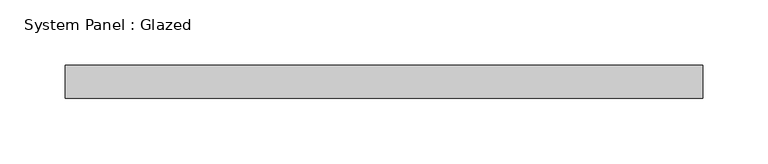
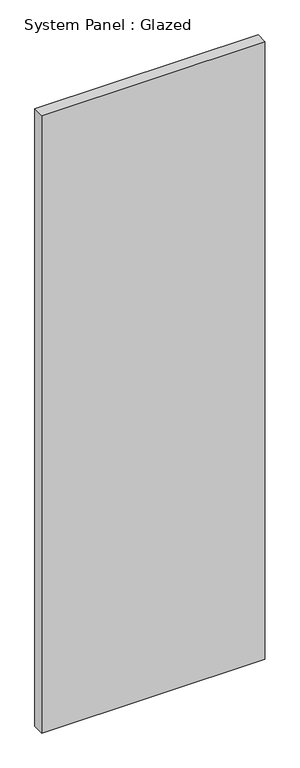
"""IFC4 building model written with IfcOpenShell, lengths in millimetres: plate geometry, System Panel : Glazed."""

from ifc_helpers import new_model, si_unit, origin, origin_with_axes, place, context, project, spatial, polyline, outline, extrude, source, transform, mapped, element, save


def system_panel_glazed_b9e07fbe(model_context):
    return source(origin(), model_context, "Body", "SweptSolid", [
        extrude(outline(polyline([(244.475, 19.05), (-244.475, 19.05), (-244.475, 44.45), (244.475, 44.45), (244.475, 19.05)])), origin_with_axes(), (0.0, 0.0, 1.0), 1429.7181357),
    ])


if __name__ == "__main__":
    model = new_model("IFC4")
    model_context = context("Model", 3, world=origin())
    ifc_project = project(units=[si_unit("LENGTHUNIT", "METRE", prefix="MILLI")], contexts=[model_context])
    site = spatial("IfcSite", under=ifc_project)
    building = spatial("IfcBuilding", under=site)
    placement = place(None, origin())
    system_panel_glazed_shape = system_panel_glazed_b9e07fbe(model_context)
    element("IfcPlate", 1, ObjectType="System Panel : Glazed", at=placement, inside=building, context=model_context, shape_type="MappedRepresentation", body=[
        mapped(system_panel_glazed_shape, transform((0.0, 0.0, 0.0), x_axis=(1.0, 0.0, 0.0), y_axis=(0.0, 1.0, 0.0), z_axis=(0.0, 0.0, 1.0))),
    ])
    save(model, "model.ifc")

# Revit data of these elements
# Type "System Panel : Glazed"
#   Construction Type Id = "GSP4R"
#   Analytic Construction = "1/8 in Pilkington single glazing"
#   Visual Light Transmittance = 0.9
#   Solar Heat Gain Coefficient = 0.86
#   Heat Transfer Coefficient (U) = 1.18115 BTU/(h·ft²·°F)
#   Define Thermal Properties by = 1
# Element 1 (IfcPlate, "System Panel : Glazed")
#   Materials on its faces: "Glass"
# Materials
#   "Glass": class "Glass", colour RGB 0 128 192, transparency 0.75, Description = "Soda Lime Glass", Cost = 0
